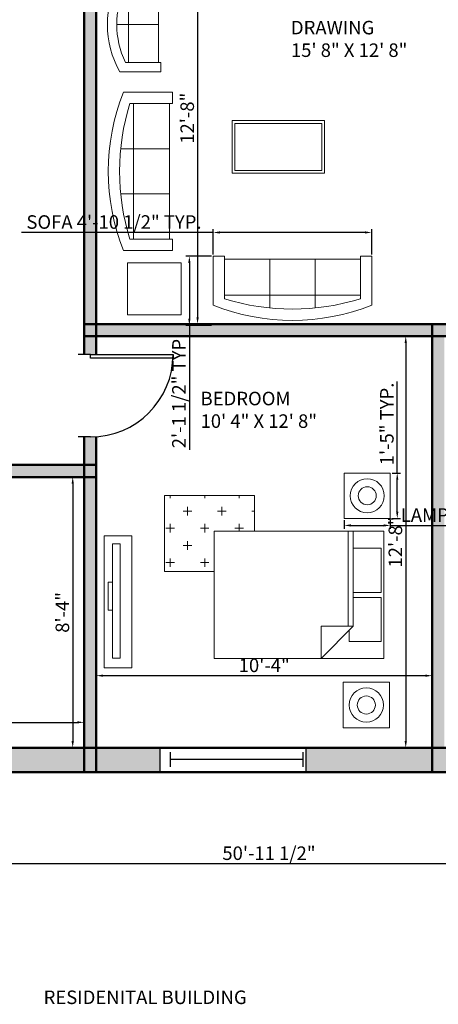
# Model space of a CAD drawing. Units: millimetres. Extents: x 3107 to 3757, y 777 to 1464.
# Tile 2 of 7: x 3324 to 3479, y 777 to 1140. Entities that reach past the tile are written whole.
import ezdxf

# ---------------------------------------------------------------- set-up
doc = ezdxf.new("R2010")
doc.units = ezdxf.units.MM
for name, color, linetype, lineweight in [('A-ANNO-DIMS', 50, 'Continuous', 18), ('A-ANNO-TEXT', 160, 'Continuous', 25), ('A-AREA-IDEN', 160, 'Continuous', 18), ('A-EQPM', 140, 'Continuous', 18), ('A-FURN-PATT', 140, 'Continuous', 13), ('A-WALL-PATT', 80, 'Continuous', 13), ('doors', 10, 'Continuous', 25), ('furniture', 140, 'Continuous', 18), ('walls', 80, 'Continuous', 50), ('windows', 30, 'Continuous', 25)]:
    doc.layers.add(name, color=color, linetype=linetype, lineweight=lineweight)
doc.styles.get("Standard").update_dxf_attribs({"font": 'arial.ttf'})
doc.dimstyles.new('ISO-25', dxfattribs={"dimtxt": 5, "dimasz": 2.5, "dimexe": 1.25, "dimexo": 0.625, "dimtad": 1, "dimdec": 0, "dimlunit": 3, "dimtxsty": 'Standard', "dimcen": 2.5, "dimadec": 0, "dimazin": 0, "dimtfac": 1, "dimtdec": 0, "dimtmove": 0, "dimatfit": 3, "dimfxl": 1, "dimarcsym": 0})

# ---------------------------------------------------------------- blocks, each defined once
blk = doc.blocks.new('*U2')
for p, q in [((0, 0), (0, -6)), ((40, 0), (40, -6))]:
    blk.add_line(p, q)
blk.add_lwpolyline([(0, 0), (0, 40), (1.75, 40), (1.75, 0)], close=True)
blk.add_arc((0, 0), 40, 0, 90)
blk = doc.blocks.new('*U4')
for p, q in [((0, 4), (0, 0)), ((36, 4), (36, 0)), ((0, 2), (36, 2))]:
    blk.add_line(p, q)
blk = doc.blocks.new('Sofa - Roundback 7 ft.')
for p, q in [((-12.00002, -32.4421), (-12.00003, -6.5971)), ((11.99997, -32.4421), (11.99998, -6.5971)), ((-36.000027, -34), (-36.000027, -11.4696)), ((-35.999844, -13.3819), (35.9998, -13.3819)), ((35.99998, -34), (35.99998, -11.4696)), ((-36.000027, -32.4421), (35.99998, -32.4421))]:
    blk.add_line(p, q)
for points in [[(-36.000027, -34), (-42.000027, -34), (-42.000027, -8)], [(41.99998, -8), (41.99998, -34), (35.99998, -34)]]:
    blk.add_lwpolyline(points)
for centre, radius, start, end in [((0, -114.25), 114.25, 68.43141, 111.5686), ((-0.00001, -127.1968), 121.1968, 72.72033, 107.2797)]:
    blk.add_arc(centre, radius, start, end)
blk = doc.blocks.new('Sofa - Roundback Loveseat 5 ft.')
for p, q in [((0, -32.44198), (0, -5.99998)), ((-24, -33.99998), (-24, -11.46958)), ((24.00004, -33.99998), (24.00004, -11.46958)), ((-23.9998, -13.38178), (23.99986, -13.38178)), ((-24, -32.44198), (24.00004, -32.44198))]:
    blk.add_line(p, q)
for points in [[(-24, -33.99998), (-30, -33.99998), (-30, -7.99998)], [(30.00004, -7.99998), (30.00004, -33.99998), (24.00004, -33.99998)]]:
    blk.add_lwpolyline(points)
for centre, radius, start, end in [((0, -60.24998), 60.24998, 60.13715, 119.8628), ((0, -61.38438), 55.38444, 64.32083, 115.6792)]:
    blk.add_arc(centre, radius, start, end)
blk = doc.blocks.new('Bed - Queen')
for p, q in [((0, -80.00003), (0, 0)), ((0, 0), (59.99999, 0)), ((59.99999, 0), (59.99999, -80.00003)), ((7.99999, -1.2), (28.79998, -1.2)), ((7.99999, -14.4), (7.99999, -1.2)), ((28.79998, -1.2), (28.79998, -14.4)), ((31.19999, -1.2), (51.99999, -1.2)), ((31.19999, -14.4), (31.19999, -1.2)), ((51.99999, -1.2), (51.99999, -16.4)), ((0, -14.4), (44.8, -14.4)), ((44.8, -16.8), (0, -16.8)), ((59.99999, -29.6), (44.8, -14.4)), ((44.8, -14.4), (44.8, -29.6)), ((51.99999, -16.4), (46.79936, -16.4)), ((44.8, -29.6), (59.99999, -29.6)), ((59.99999, -80.00003), (0, -80.00003))]:
    blk.add_line(p, q)
blk = doc.blocks.new('*D36')
at = {"layer": 'A-ANNO-DIMS', "color": 0, "lineweight": -2, "transparency": 16777216}
for p, q in [((3344.41, 971.43), (3345.04, 971.43)), ((3343.79, 968.93), (3343.79, 873.93)), ((3344.41, 871.43), (3345.04, 871.43))]:
    blk.add_line(p, q, dxfattribs=at)
at = {"layer": 'A-ANNO-DIMS', "color": 0, "transparency": 16777216}
for points in [[(3343.37, 968.93), (3344.21, 968.93), (3343.79, 971.43)], [(3343.37, 873.93), (3344.21, 873.93), (3343.79, 871.43)]]:
    blk.add_solid(points, dxfattribs=at)
at = {"layer": 'Defpoints', "color": 0, "transparency": 16777216}
for p in [(3343.79, 971.43), (3343.79, 871.43), (3343.79, 871.43)]:
    blk.add_point(p, dxfattribs=at)
at = {"layer": 'A-ANNO-DIMS', "color": 0, "transparency": 16777216, "insert": (3340.61, 921.43), "char_height": 5, "attachment_point": 5, "rotation": 90}
blk.add_mtext('8\'-4"', dxfattribs=at)
blk = doc.blocks.new('*D37')
at = {"layer": 'A-ANNO-DIMS', "color": 0, "lineweight": -2, "transparency": 16777216}
for p, q in [((3271.97, 881.46), (3271.97, 882.08)), ((3274.47, 880.83), (3345.47, 880.83)), ((3347.97, 881.46), (3347.97, 882.08))]:
    blk.add_line(p, q, dxfattribs=at)
at = {"layer": 'A-ANNO-DIMS', "color": 0, "transparency": 16777216}
for points in [[(3274.47, 881.25), (3274.47, 880.41), (3271.97, 880.83)], [(3345.47, 881.25), (3345.47, 880.41), (3347.97, 880.83)]]:
    blk.add_solid(points, dxfattribs=at)
at = {"layer": 'Defpoints', "color": 0, "transparency": 16777216}
for p in [(3271.97, 880.83), (3347.97, 880.83), (3347.97, 880.83)]:
    blk.add_point(p, dxfattribs=at)
at = {"layer": 'A-ANNO-DIMS', "color": 0, "transparency": 16777216, "insert": (3309.97, 884.01), "char_height": 5, "attachment_point": 5}
blk.add_mtext('6\'-4"', dxfattribs=at)
blk = doc.blocks.new('*D38')
at = {"layer": 'A-ANNO-DIMS', "color": 0, "lineweight": -2, "transparency": 16777216}
for p, q in [((3352.47, 899.15), (3352.47, 896.81)), ((3476.47, 899.15), (3476.47, 896.81)), ((3473.97, 898.06), (3354.97, 898.06))]:
    blk.add_line(p, q, dxfattribs=at)
at = {"layer": 'A-ANNO-DIMS', "color": 0, "transparency": 16777216}
for points in [[(3354.97, 898.48), (3354.97, 897.65), (3352.47, 898.06)], [(3473.97, 898.48), (3473.97, 897.65), (3476.47, 898.06)]]:
    blk.add_solid(points, dxfattribs=at)
at = {"layer": 'Defpoints', "color": 0, "transparency": 16777216}
for p in [(3352.47, 899.77), (3476.47, 899.77), (3352.47, 898.06)]:
    blk.add_point(p, dxfattribs=at)
at = {"layer": 'A-ANNO-DIMS', "color": 0, "transparency": 16777216, "insert": (3414.47, 901.24), "char_height": 5, "attachment_point": 5}
blk.add_mtext('10\'-4"', dxfattribs=at)
blk = doc.blocks.new('*D39')
at = {"layer": 'A-ANNO-DIMS', "color": 0, "lineweight": -2, "transparency": 16777216}
for p, q in [((3470.35, 1023.43), (3465.45, 1023.43)), ((3466.7, 1020.93), (3466.7, 873.93)), ((3472.66, 871.43), (3465.45, 871.43))]:
    blk.add_line(p, q, dxfattribs=at)
at = {"layer": 'A-ANNO-DIMS', "color": 0, "transparency": 16777216}
for points in [[(3466.28, 1020.93), (3467.12, 1020.93), (3466.7, 1023.43)], [(3466.28, 873.93), (3467.12, 873.93), (3466.7, 871.43)]]:
    blk.add_solid(points, dxfattribs=at)
at = {"layer": 'Defpoints', "color": 0, "transparency": 16777216}
for p in [(3470.97, 1023.43), (3466.7, 871.43), (3473.29, 871.43)]:
    blk.add_point(p, dxfattribs=at)
at = {"layer": 'A-ANNO-DIMS', "color": 0, "transparency": 16777216, "insert": (3463.52, 947.43), "char_height": 5, "attachment_point": 5, "rotation": 90}
blk.add_mtext('12\'-8"', dxfattribs=at)
blk = doc.blocks.new('*D40')
at = {"layer": 'A-ANNO-DIMS', "color": 0, "lineweight": -2, "transparency": 16777216}
for p, q in [((3385.8, 1179.93), (3391.12, 1179.93)), ((3389.87, 1177.43), (3389.87, 1030.43)), ((3384.41, 1027.93), (3391.12, 1027.93))]:
    blk.add_line(p, q, dxfattribs=at)
at = {"layer": 'A-ANNO-DIMS', "color": 0, "transparency": 16777216}
for points in [[(3389.45, 1177.43), (3390.29, 1177.43), (3389.87, 1179.93)], [(3389.45, 1030.43), (3390.29, 1030.43), (3389.87, 1027.93)]]:
    blk.add_solid(points, dxfattribs=at)
at = {"layer": 'Defpoints', "color": 0, "transparency": 16777216}
for p in [(3385.18, 1179.93), (3383.78, 1027.93), (3389.87, 1027.93)]:
    blk.add_point(p, dxfattribs=at)
at = {"layer": 'A-ANNO-DIMS', "color": 0, "transparency": 16777216, "insert": (3386.69, 1103.93), "char_height": 5, "attachment_point": 5, "rotation": 90}
blk.add_mtext('12\'-8"', dxfattribs=at)
blk = doc.blocks.new('BEDSIDE-TABLE-LAMP')
blk.add_lwpolyline([(17.05, 16.79), (0, 16.79), (0, 0), (17.05, 0)], close=True)
for radius in [6.29, 3.33]:
    blk.add_circle((8.52, 8.4), radius)
blk = doc.blocks.new('*D55')
at = {"layer": 'A-ANNO-DIMS', "color": 0, "lineweight": -2, "transparency": 16777216}
for p, q in [((3395.62, 1053.59), (3395.62, 1062.99)), ((3454.14, 1053.59), (3454.14, 1062.99)), ((3395.62, 1061.74), (3324.92, 1061.74)), ((3451.64, 1061.74), (3398.12, 1061.74))]:
    blk.add_line(p, q, dxfattribs=at)
at = {"layer": 'A-ANNO-DIMS', "color": 0, "transparency": 16777216}
for points in [[(3398.12, 1062.16), (3398.12, 1061.33), (3395.62, 1061.74)], [(3451.64, 1062.16), (3451.64, 1061.33), (3454.14, 1061.74)]]:
    blk.add_solid(points, dxfattribs=at)
at = {"layer": 'Defpoints', "color": 0, "transparency": 16777216}
for p in [(3395.62, 1061.74), (3395.62, 1052.96), (3454.14, 1052.96)]:
    blk.add_point(p, dxfattribs=at)
at = {"layer": 'A-ANNO-DIMS', "color": 0, "transparency": 16777216, "insert": (3359.02, 1064.95), "char_height": 5, "attachment_point": 5}
blk.add_mtext('SOFA 4\'-10 1/2" TYP.', dxfattribs=at)
blk = doc.blocks.new('*D56')
at = {"layer": 'A-ANNO-DIMS', "color": 0, "lineweight": -2, "transparency": 16777216}
for p, q in [((3394.99, 1052.96), (3385.59, 1052.96)), ((3386.84, 1050.46), (3386.84, 1029.92)), ((3394.99, 1027.42), (3385.59, 1027.42)), ((3386.84, 1027.42), (3386.84, 981.45))]:
    blk.add_line(p, q, dxfattribs=at)
at = {"layer": 'A-ANNO-DIMS', "color": 0, "transparency": 16777216}
for points in [[(3386.42, 1050.46), (3387.26, 1050.46), (3386.84, 1052.96)], [(3386.42, 1029.92), (3387.26, 1029.92), (3386.84, 1027.42)]]:
    blk.add_solid(points, dxfattribs=at)
at = {"layer": 'Defpoints', "color": 0, "transparency": 16777216}
for p in [(3395.62, 1052.96), (3386.84, 1027.42), (3395.62, 1027.42)]:
    blk.add_point(p, dxfattribs=at)
at = {"layer": 'A-ANNO-DIMS', "color": 0, "transparency": 16777216, "insert": (3383.63, 1003.19), "char_height": 5, "attachment_point": 5, "rotation": 90}
blk.add_mtext('2\'-1 1/2" TYP.', dxfattribs=at)
blk = doc.blocks.new('*D63')
at = {"layer": 'A-ANNO-DIMS', "color": 0, "lineweight": -2, "transparency": 16777216}
for p, q in [((3443.96, 955.48), (3443.96, 952.3)), ((3446.46, 953.55), (3458.5, 953.55)), ((3461, 955.48), (3461, 952.3)), ((3461, 953.55), (3515.97, 953.55))]:
    blk.add_line(p, q, dxfattribs=at)
at = {"layer": 'A-ANNO-DIMS', "color": 0, "transparency": 16777216}
for points in [[(3446.46, 953.96), (3446.46, 953.13), (3443.96, 953.55)], [(3458.5, 953.96), (3458.5, 953.13), (3461, 953.55)]]:
    blk.add_solid(points, dxfattribs=at)
at = {"layer": 'Defpoints', "color": 0, "transparency": 16777216}
for p in [(3443.96, 956.1), (3461, 956.1), (3461, 953.55)]:
    blk.add_point(p, dxfattribs=at)
at = {"layer": 'A-ANNO-DIMS', "color": 0, "transparency": 16777216, "insert": (3489.74, 956.72), "char_height": 5, "attachment_point": 5}
blk.add_mtext('LAMP 1\'-5" TYP.', dxfattribs=at)
blk = doc.blocks.new('*D64')
at = {"layer": 'A-ANNO-DIMS', "color": 0, "lineweight": -2, "transparency": 16777216}
for p, q in [((3463.56, 972.89), (3463.56, 1006.65)), ((3461.63, 972.89), (3464.81, 972.89)), ((3463.56, 958.6), (3463.56, 970.39)), ((3461.63, 956.1), (3464.81, 956.1))]:
    blk.add_line(p, q, dxfattribs=at)
at = {"layer": 'A-ANNO-DIMS', "color": 0, "transparency": 16777216}
for points in [[(3463.15, 970.39), (3463.98, 970.39), (3463.56, 972.89)], [(3463.15, 958.6), (3463.98, 958.6), (3463.56, 956.1)]]:
    blk.add_solid(points, dxfattribs=at)
at = {"layer": 'Defpoints', "color": 0, "transparency": 16777216}
for p in [(3461, 972.89), (3463.56, 972.89), (3461, 956.1)]:
    blk.add_point(p, dxfattribs=at)
at = {"layer": 'A-ANNO-DIMS', "color": 0, "transparency": 16777216, "insert": (3460.38, 991.02), "char_height": 5, "attachment_point": 5, "rotation": 90}
blk.add_mtext('1\'-5" TYP.', dxfattribs=at)
blk = doc.blocks.new('*D69')
at = {"layer": 'A-ANNO-DIMS', "color": 0, "lineweight": -2, "transparency": 16777216}
for p, q in [((3110.47, 861.8), (3110.47, 827.39)), ((3721.97, 861.8), (3721.97, 827.39)), ((3112.97, 828.64), (3719.47, 828.64))]:
    blk.add_line(p, q, dxfattribs=at)
at = {"layer": 'A-ANNO-DIMS', "color": 0, "transparency": 16777216}
for points in [[(3112.97, 829.06), (3112.97, 828.22), (3110.47, 828.64)], [(3719.47, 829.06), (3719.47, 828.22), (3721.97, 828.64)]]:
    blk.add_solid(points, dxfattribs=at)
at = {"layer": 'Defpoints', "color": 0, "transparency": 16777216}
for p in [(3110.47, 862.43), (3721.97, 862.43), (3721.97, 828.64)]:
    blk.add_point(p, dxfattribs=at)
at = {"layer": 'A-ANNO-DIMS', "color": 0, "transparency": 16777216, "insert": (3416.22, 831.85), "char_height": 5, "attachment_point": 5}
blk.add_mtext('50\'-11 1/2"', dxfattribs=at)

msp = doc.modelspace()

# ---------------------------------------------------------------- hatches: boundary and pattern name
at = {"layer": 'A-FURN-PATT'}
h = msp.add_hatch(dxfattribs=at)
h.set_pattern_fill('CROSS', color=256)
h.paths.add_polyline_path([(3395.95, 951.39), (3410.87, 951.39), (3410.87, 964.57), (3377.69, 964.57), (3377.69, 936.51), (3395.95, 936.51)])
at = {"layer": 'A-WALL-PATT'}
h = msp.add_hatch(color=256, dxfattribs=at)
h.dxf.hatch_style = 1
h.paths.add_polyline_path([(3119.47, 1087.39), (3110.47, 1087.39), (3110.47, 1027.93), (3119.47, 1027.93)])
h.paths.add_polyline_path([(3119.47, 1027.93), (3110.47, 1027.93), (3110.47, 1023.43), (3119.47, 1023.43)])
h.paths.add_polyline_path([(3267.47, 1027.93), (3119.47, 1027.93), (3119.47, 1023.43), (3267.47, 1023.43)])
h.paths.add_polyline_path([(3119.47, 1023.43), (3110.47, 1023.43), (3110.47, 979.44), (3119.47, 979.44)])
h.paths.add_polyline_path([(3299.97, 1179.93), (3295.47, 1179.93), (3295.47, 1027.93), (3299.97, 1027.93)])
h.paths.add_polyline_path([(3295.47, 1027.93), (3271.97, 1027.93), (3271.97, 1023.43), (3295.47, 1023.43)])
h.paths.add_polyline_path([(3271.97, 1027.93), (3267.47, 1027.93), (3267.47, 1023.43), (3271.97, 1023.43)])
h.paths.add_polyline_path([(3299.97, 1027.93), (3295.47, 1027.93), (3295.47, 1023.43), (3299.97, 1023.43)])
h.paths.add_polyline_path([(3299.97, 1184.43), (3295.47, 1184.43), (3295.47, 1179.93), (3299.97, 1179.93)])
h.paths.add_polyline_path([(3295.47, 1184.43), (3288.38, 1184.43), (3288.38, 1182.47), (3288.38, 1179.93), (3295.47, 1179.93)])
h.paths.add_polyline_path([(3352.47, 1179.93), (3347.97, 1179.93), (3347.97, 1027.93), (3352.47, 1027.93)])
h.paths.add_polyline_path([(3352.47, 1184.43), (3347.97, 1184.43), (3347.97, 1179.93), (3352.47, 1179.93)])
h.paths.add_polyline_path([(3464.47, 1184.43), (3352.47, 1184.43), (3352.47, 1179.93), (3464.47, 1179.93)])
h.paths.add_polyline_path([(3468.97, 1288.93), (3464.47, 1288.93), (3464.47, 1184.43), (3468.97, 1184.43)])
h.paths.add_polyline_path([(3468.97, 1184.43), (3464.47, 1184.43), (3464.47, 1179.93), (3468.97, 1179.93)])
h.paths.add_polyline_path([(3195.97, 1248.43), (3191.47, 1248.43), (3191.47, 1184.43), (3195.97, 1184.43)])
h.paths.add_polyline_path([(3195.97, 1184.43), (3191.47, 1184.43), (3191.47, 1179.93), (3195.97, 1179.93)])
h.paths.add_polyline_path([(3191.47, 1184.43), (3183.28, 1184.43), (3183.28, 1181.58), (3183.28, 1179.93), (3191.47, 1179.93)])
h.paths.add_polyline_path([(3243.97, 1184.43), (3195.97, 1184.43), (3195.97, 1179.93), (3243.97, 1179.93)])
h.paths.add_polyline_path([(3257.91, 1182.47), (3257.91, 1184.43), (3248.47, 1184.43), (3248.47, 1179.93), (3258.02, 1179.93, -0.020891)])
h.paths.add_polyline_path([(3248.47, 1184.43), (3243.97, 1184.43), (3243.97, 1179.93), (3248.47, 1179.93)])
h.paths.add_polyline_path([(3248.47, 1189.24), (3247.51, 1189.24), (3243.97, 1189.24), (3243.97, 1184.43), (3248.47, 1184.43)])
h.paths.add_polyline_path([(3166.87, 1184.43), (3119.47, 1184.43), (3119.47, 1179.93), (3166.63, 1179.93), (3166.63, 1181.58, -0.042981)])
h.paths.add_polyline_path([(3119.47, 1184.43), (3110.47, 1184.43), (3110.47, 1179.93), (3119.47, 1179.93)])
h.paths.add_polyline_path([(3119.47, 1248.43), (3110.47, 1248.43), (3110.47, 1184.43), (3119.47, 1184.43)])
h.paths.add_polyline_path([(3119.47, 1179.93), (3110.47, 1179.93), (3110.47, 1140.65), (3119.47, 1140.65)])
h.paths.add_polyline_path([(3119.47, 1288.93), (3110.47, 1288.93), (3110.47, 1252.93), (3119.47, 1252.93)])
h.paths.add_polyline_path([(3119.47, 1252.93), (3110.47, 1252.93), (3110.47, 1248.43), (3119.47, 1248.43)])
h.paths.add_polyline_path([(3191.47, 1252.93), (3119.47, 1252.93), (3119.47, 1248.43), (3191.47, 1248.43)])
h.paths.add_polyline_path([(3195.97, 1288.93), (3191.47, 1288.93), (3191.47, 1252.93), (3195.97, 1252.93)])
h.paths.add_polyline_path([(3195.97, 1252.93), (3191.47, 1252.93), (3191.47, 1248.43), (3195.97, 1248.43)])
h.paths.add_polyline_path([(3248.47, 1293.43), (3243.97, 1293.43), (3243.97, 1288.93), (3248.47, 1288.93)])
h.paths.add_polyline_path([(3243.97, 1293.43), (3195.97, 1293.43), (3195.97, 1288.93), (3243.97, 1288.93)])
h.paths.add_polyline_path([(3303.47, 1293.43), (3248.47, 1293.43), (3248.47, 1288.93), (3303.47, 1288.93)])
h.paths.add_polyline_path([(3248.47, 1288.93), (3243.97, 1288.93), (3243.97, 1205.51, -0.053712), (3247.51, 1205.89), (3248.47, 1205.89)])
h.paths.add_polyline_path([(3191.47, 1293.43), (3119.47, 1293.43), (3119.47, 1288.93), (3191.47, 1288.93)])
h.paths.add_polyline_path([(3119.47, 1293.43), (3110.47, 1293.43), (3110.47, 1288.93), (3119.47, 1288.93)])
h.paths.add_polyline_path([(3119.47, 1322.96, -0.065064), (3111.64, 1321.93), (3110.47, 1321.93), (3110.47, 1293.43), (3119.47, 1293.43)])
h.paths.add_polyline_path([(3195.97, 1293.43), (3191.47, 1293.43), (3191.47, 1288.93), (3195.97, 1288.93)])
h.paths.add_polyline_path([(3119.47, 1450.43), (3110.47, 1450.43), (3110.47, 1441.43), (3119.47, 1441.43)])
h.paths.add_polyline_path([(3119.47, 1441.43), (3110.47, 1441.43), (3110.47, 1352.4), (3111.64, 1352.4), (3119.47, 1352.4)])
h.paths.add_polyline_path([(3176.58, 1450.43), (3119.47, 1450.43), (3119.47, 1441.43), (3176.58, 1441.43)])
h.paths.add_polyline_path([(3323.19, 1450.43), (3307.97, 1450.43), (3307.97, 1441.43), (3323.19, 1441.43)])
h.paths.add_polyline_path([(3307.97, 1450.43), (3303.47, 1450.43), (3303.47, 1441.43), (3307.97, 1441.43)])
h.paths.add_polyline_path([(3303.47, 1450.43), (3229.4, 1450.43), (3229.4, 1441.43), (3303.47, 1441.43)])
h.paths.add_polyline_path([(3307.97, 1441.43), (3303.47, 1441.43), (3303.47, 1363.43), (3307.97, 1363.43)])
h.paths.add_polyline_path([(3307.97, 1363.43), (3303.47, 1363.43), (3303.47, 1358.93), (3307.97, 1358.93)])
h.paths.add_polyline_path([(3307.97, 1358.93), (3303.47, 1358.93), (3303.47, 1342.3), (3305.5, 1342.3, -0.037178), (3307.97, 1342.12)])
h.paths.add_polyline_path([(3379.97, 1363.43), (3307.97, 1363.43), (3307.97, 1358.93), (3379.97, 1358.93)])
h.paths.add_polyline_path([(3384.47, 1393.61), (3383.04, 1393.61), (3379.97, 1393.61), (3379.97, 1363.43), (3384.47, 1363.43)])
h.paths.add_polyline_path([(3384.47, 1363.43), (3379.97, 1363.43), (3379.97, 1358.93), (3384.47, 1358.93)])
h.paths.add_polyline_path([(3384.47, 1358.93), (3379.97, 1358.93), (3379.97, 1293.43), (3384.47, 1293.43)])
h.paths.add_polyline_path([(3384.47, 1441.43), (3379.97, 1441.43), (3379.97, 1409.98, -0.046389), (3383.04, 1410.27), (3384.47, 1410.27)])
h.paths.add_polyline_path([(3384.47, 1450.43), (3379.97, 1450.43), (3379.97, 1441.43), (3384.47, 1441.43)])
h.paths.add_polyline_path([(3379.97, 1450.43), (3357.18, 1450.43), (3357.18, 1441.43), (3379.97, 1441.43)])
h.paths.add_polyline_path([(3432.79, 1450.43), (3384.47, 1450.43), (3384.47, 1441.43), (3432.79, 1441.43)])
h.paths.add_polyline_path([(3540.47, 1450.43), (3484.18, 1450.43), (3484.18, 1441.43), (3540.47, 1441.43)])
h.paths.add_polyline_path([(3544.97, 1450.43), (3540.47, 1450.43), (3540.47, 1441.43), (3544.97, 1441.43)])
h.paths.add_polyline_path([(3544.97, 1441.43), (3540.47, 1441.43), (3540.47, 1293.43), (3544.97, 1293.43)])
h.paths.add_polyline_path([(3590.83, 1450.43), (3544.97, 1450.43), (3544.97, 1441.43), (3590.83, 1441.43)])
h.paths.add_polyline_path([(3712.97, 1450.43), (3645.62, 1450.43), (3645.62, 1441.43), (3712.97, 1441.43)])
h.paths.add_polyline_path([(3721.97, 1441.43), (3712.97, 1441.43), (3712.97, 1288.93), (3712.97, 1184.43), (3721.97, 1184.43), (3721.97, 1288.93)])
h.paths.add_polyline_path([(3721.97, 1450.43), (3712.97, 1450.43), (3712.97, 1441.43), (3721.97, 1441.43)])
h.paths.add_polyline_path([(3712.97, 1184.43), (3658.24, 1184.43), (3658.24, 1183.15), (3658.24, 1179.93), (3712.97, 1179.93)])
h.paths.add_polyline_path([(3721.97, 1184.43), (3712.97, 1184.43), (3712.97, 1179.93), (3721.97, 1179.93)])
h.paths.add_polyline_path([(3597.32, 1183.15), (3597.32, 1184.43), (3544.97, 1184.43), (3544.97, 1179.93), (3597.32, 1179.93)])
h.paths.add_polyline_path([(3544.97, 1184.43), (3540.47, 1184.43), (3540.47, 1179.93), (3544.97, 1179.93)])
h.paths.add_polyline_path([(3544.97, 1179.93), (3540.47, 1179.93), (3540.47, 1143.69), (3543.65, 1143.69), (3544.97, 1143.69)])
h.paths.add_polyline_path([(3721.97, 1179.93), (3712.97, 1179.93), (3712.97, 1006.22), (3712.97, 871.43), (3721.97, 871.43), (3721.97, 1006.22)])
h.paths.add_polyline_path([(3468.97, 1293.43), (3464.47, 1293.43), (3464.47, 1288.93), (3468.97, 1288.93)])
h.paths.add_polyline_path([(3540.47, 1293.43), (3468.97, 1293.43), (3468.97, 1288.93), (3540.47, 1288.93)])
h.paths.add_polyline_path([(3544.97, 1293.43), (3540.47, 1293.43), (3540.47, 1288.93), (3544.97, 1288.93)])
h.paths.add_polyline_path([(3464.47, 1293.43), (3417.83, 1293.43, -0.015057), (3417.88, 1291.6), (3417.88, 1288.93), (3464.47, 1288.93)])
h.paths.add_polyline_path([(3379.97, 1293.43), (3307.97, 1293.43), (3307.97, 1288.93), (3379.97, 1288.93)])
h.paths.add_polyline_path([(3307.97, 1325.65), (3305.5, 1325.65), (3303.47, 1325.65), (3303.47, 1293.43), (3307.97, 1293.43)])
h.paths.add_polyline_path([(3307.97, 1293.43), (3303.47, 1293.43), (3303.47, 1288.93), (3307.97, 1288.93)])
h.paths.add_polyline_path([(3384.47, 1293.43), (3379.97, 1293.43), (3379.97, 1288.93), (3384.47, 1288.93)])
h.paths.add_polyline_path([(3387.42, 1291.6), (3387.42, 1293.43), (3384.47, 1293.43), (3384.47, 1288.93), (3387.42, 1288.93)])
h.paths.add_polyline_path([(3119.47, 927.28), (3110.47, 927.28), (3110.47, 871.43), (3119.47, 871.43)])
h.paths.add_polyline_path([(3119.47, 871.43), (3110.47, 871.43), (3110.47, 862.43), (3119.47, 862.43)])
h.paths.add_polyline_path([(3267.47, 871.43), (3119.47, 871.43), (3119.47, 862.43), (3267.47, 862.43)])
h.paths.add_polyline_path([(3271.97, 971.43), (3267.47, 971.43), (3267.47, 871.43), (3271.97, 871.43)])
h.paths.add_polyline_path([(3271.97, 871.43), (3267.47, 871.43), (3267.47, 862.43), (3271.97, 862.43)])
h.paths.add_polyline_path([(3287.13, 871.43), (3271.97, 871.43), (3271.97, 862.43), (3287.13, 862.43)])
h.paths.add_polyline_path([(3347.97, 871.43), (3318.96, 871.43), (3318.96, 862.43), (3347.97, 862.43)])
h.paths.add_polyline_path([(3352.47, 971.43), (3347.97, 971.43), (3347.97, 871.43), (3352.47, 871.43)])
h.paths.add_polyline_path([(3352.47, 871.43), (3347.97, 871.43), (3347.97, 862.43), (3352.47, 862.43)])
h.paths.add_polyline_path([(3375.96, 871.43), (3352.47, 871.43), (3352.47, 862.43), (3375.96, 862.43)])
h.paths.add_polyline_path([(3352.47, 975.93), (3347.97, 975.93), (3347.97, 971.43), (3352.47, 971.43)])
h.paths.add_polyline_path([(3352.47, 986.27, -0.01722), (3350.37, 986.2), (3347.97, 986.2), (3347.97, 975.93), (3352.47, 975.93)])
h.paths.add_polyline_path([(3347.97, 975.93), (3292.38, 975.93), (3292.38, 973.47, -0.030785), (3292.25, 971.43), (3347.97, 971.43)])
h.paths.add_polyline_path([(3271.97, 985.98), (3269.95, 985.98), (3267.47, 985.98), (3267.47, 975.93), (3271.97, 975.93)])
h.paths.add_polyline_path([(3271.97, 975.93), (3267.47, 975.93), (3267.47, 971.43), (3271.97, 971.43)])
h.paths.add_polyline_path([(3275.72, 975.93), (3271.97, 975.93), (3271.97, 971.43), (3275.72, 971.43), (3275.72, 973.47)])
h.paths.add_polyline_path([(3271.97, 1023.43), (3267.47, 1023.43), (3267.47, 1016.34, -0.020418), (3269.95, 1016.44), (3271.97, 1016.44)])
h.paths.add_polyline_path([(3352.47, 1023.43), (3347.97, 1023.43), (3347.97, 1016.67), (3350.37, 1016.67), (3352.47, 1016.67)])
h.paths.add_polyline_path([(3352.47, 1027.93), (3347.97, 1027.93), (3347.97, 1023.43), (3352.47, 1023.43)])
h.paths.add_polyline_path([(3476.47, 1027.93), (3352.47, 1027.93), (3352.47, 1023.43), (3476.47, 1023.43)])
h.paths.add_polyline_path([(3540.47, 1027.93), (3480.97, 1027.93), (3480.97, 1023.43), (3540.47, 1023.43)])
h.paths.add_polyline_path([(3480.97, 1027.93), (3476.47, 1027.93), (3476.47, 1023.43), (3480.97, 1023.43)])
h.paths.add_polyline_path([(3480.97, 1023.43), (3476.47, 1023.43), (3476.47, 871.43), (3480.97, 871.43)])
h.paths.add_polyline_path([(3476.47, 871.43), (3429.88, 871.43), (3429.88, 862.43), (3476.47, 862.43)])
h.paths.add_polyline_path([(3480.97, 871.43), (3476.47, 871.43), (3476.47, 862.43), (3480.97, 862.43)])
h.paths.add_polyline_path([(3493.81, 871.43), (3480.97, 871.43), (3480.97, 862.43), (3493.81, 862.43)])
h.paths.add_polyline_path([(3712.97, 871.43), (3525.61, 871.43), (3525.61, 862.43), (3712.97, 862.43)])
h.paths.add_polyline_path([(3721.97, 871.43), (3712.97, 871.43), (3712.97, 862.43), (3721.97, 862.43)])

# ---------------------------------------------------------------- linework, layer by layer
at = {"layer": 'A-EQPM'}
for points in [[(3355.44, 949.76), (3365.61, 949.76), (3365.61, 901), (3355.44, 901)], [(3358.52, 946.76), (3361.24, 946.76), (3361.24, 904.54), (3358.52, 904.54)], [(3358.52, 932.58), (3356.93, 932.58), (3356.93, 922.22), (3358.52, 922.22)]]:
    msp.add_lwpolyline(points, close=True, dxfattribs=at)
at = {"layer": 'furniture'}
for p, q in [((3377.69, 936.51), (3377.69, 964.57)), ((3377.69, 964.57), (3410.87, 964.57)), ((3410.87, 964.57), (3410.87, 951.39)), ((3395.95, 936.51), (3377.69, 936.51))]:
    msp.add_line(p, q, dxfattribs=at)
for points in [[(3402.68, 1083.63), (3402.68, 1103.03), (3436.67, 1103.03), (3436.67, 1083.63)], [(3403.68, 1084.63), (3403.68, 1102.03), (3435.67, 1102.03), (3435.67, 1084.63)], [(3363.99, 1050.54), (3383.78, 1050.54), (3383.78, 1031.32), (3363.99, 1031.32)]]:
    msp.add_lwpolyline(points, close=True, dxfattribs=at)
at = {"layer": 'walls'}
for p, q in [((3347.97, 1184.43), (3347.97, 1016.67)), ((3352.47, 1184.43), (3352.47, 1016.67)), ((3347.97, 1027.93), (3544.97, 1027.93)), ((3476.47, 1027.93), (3476.47, 862.43)), ((3347.97, 1023.43), (3544.97, 1023.43)), ((3347.97, 986.2), (3347.97, 862.43)), ((3352.47, 986.27), (3352.47, 862.43)), ((3292.38, 975.93), (3352.47, 975.93)), ((3292.25, 971.43), (3352.47, 971.43)), ((3110.47, 871.43), (3721.97, 871.43)), ((3110.47, 862.43), (3721.97, 862.43))]:
    msp.add_line(p, q, dxfattribs=at)
at = {"layer": 'windows'}
for p, q in [((3375.96, 871.43), (3375.96, 862.43)), ((3429.88, 871.43), (3429.88, 862.43))]:
    msp.add_line(p, q, dxfattribs=at)

# ---------------------------------------------------------------- block references
at = {"layer": 'doors', "xscale": 0.7615706373352984, "yscale": 0.7615706373352984, "zscale": 0.7615706373352984, "rotation": 269.9999999999999}
msp.add_blockref('*U2', (3350.37, 1016.67), dxfattribs=at)
at = {"layer": 'furniture'}
for name, p, xscale, yscale, zscale, rotation in [('Sofa - Roundback Loveseat 5 ft.', (3356.57, 1138.5), 0.5809767439628069, 0.5809767439628069, 0.5809767439628069, 89.99996919953323), ('Sofa - Roundback 7 ft.', (3356.91, 1084.32), 0.6967080671381904, 0.6967080671381904, 0.6967080671381904, 90), ('Sofa - Roundback 7 ft.', (3424.88, 1029.28), 0.6967080671381904, 0.6967080671381904, 0.6967080671381904, 180), ('Bed - Queen', (3458.63, 951.39), 0.7835133119924312, 0.7835133119924312, 0.7835133119924312, 270)]:
    msp.add_blockref(name, p, dxfattribs=dict(at, xscale=xscale, yscale=yscale, zscale=zscale, rotation=rotation))
for p in [(3443.96, 956.1), (3443.63, 878.83)]:
    msp.add_blockref('BEDSIDE-TABLE-LAMP', p, dxfattribs=at)
at = {"layer": 'windows', "xscale": 1.357941570966636, "yscale": 1.357941570966636, "zscale": 1.357941570966636, "rotation": 180}
msp.add_blockref('*U4', (3428.79, 869.87), dxfattribs=at)

# ---------------------------------------------------------------- texts
at = {"layer": 'A-ANNO-TEXT', "insert": (3333.05, 781.79), "char_height": 5, "attachment_point": 1}
msp.add_mtext_dynamic_manual_height_columns('RESIDENITAL BUILDING ', width=274.8882, gutter_width=12.5, heights=[0], dxfattribs=at)
at = {"layer": 'A-AREA-IDEN', "char_height": 5, "attachment_point": 1}
for s, width, insert in [('DRAWING \\P15\' 8" X 12\' 8"', 62.5375, (3424.32, 1139.89)), ('BEDROOM\\P10\' 4" X 12\' 8"', 61.2307, (3390.97, 1002.91))]:
    msp.add_mtext_dynamic_manual_height_columns(s, width=width, gutter_width=12.5, heights=[0], dxfattribs=dict(at, insert=insert))

# ---------------------------------------------------------------- dimensions: what is measured, and where the dimension line sits
at = {"layer": 'A-ANNO-DIMS'}
for base, p1, p2, picture, middle in [((3389.87, 1027.93), (3385.18, 1179.93), (3383.78, 1027.93), '*D40', (3386.69, 1103.93)), ((3466.7, 871.43), (3470.97, 1023.43), (3473.29, 871.43), '*D39', (3463.52, 947.43)), ((3343.79, 871.43), (3343.79, 971.43), (3343.79, 871.43), '*D36', (3340.61, 921.43))]:
    dim = msp.add_linear_dim(base=base, p1=p1, p2=p2, angle=90, dimstyle='ISO-25', override={"dimclrd": 0, "dimclre": 0, "dimclrt": 0}, dxfattribs=at)
    dim.commit()
    dim.dimension.update_dxf_attribs({"geometry": picture, "text_midpoint": middle})
for base, p1, p2, angle, text, picture, middle in [((3395.62, 1061.74), (3454.14, 1052.96), (3395.62, 1052.96), 180, 'SOFA <> TYP.', '*D55', (3359.02, 1064.95)), ((3386.84, 1027.42), (3395.62, 1052.96), (3395.62, 1027.42), 270, '<> TYP.', '*D56', (3383.63, 1003.19)), ((3463.56, 972.89), (3461, 956.1), (3461, 972.89), 90, '<> TYP.', '*D64', (3460.38, 991.02))]:
    dim = msp.add_linear_dim(base=base, p1=p1, p2=p2, angle=angle, text=text, dimstyle='ISO-25', override={"dimdec": 1, "dimlfac": 1, "dimrnd": 0, "dimzin": 1, "dimdsep": 46, "dimlunit": 4, "dimfrac": 2}, dxfattribs=at)
    dim.commit()
    dim.dimension.update_dxf_attribs({"geometry": picture, "text_midpoint": middle})
dim = msp.add_linear_dim(base=(3461, 953.55), p1=(3443.96, 956.1), p2=(3461, 956.1), text='LAMP <> TYP.', dimstyle='ISO-25', override={"dimdec": 1, "dimlfac": 1, "dimrnd": 0, "dimzin": 1, "dimdsep": 46, "dimlunit": 4, "dimfrac": 2}, dxfattribs=at)
dim.commit()
dim.dimension.update_dxf_attribs({"geometry": '*D63', "text_midpoint": (3489.74, 956.72)})
for base, p1, p2, override, picture, middle in [((3352.47, 898.06), (3476.47, 899.77), (3352.47, 899.77), {"dimclrd": 0, "dimclre": 0, "dimclrt": 0}, '*D38', (3414.47, 901.24)), ((3347.97, 880.83), (3271.97, 880.83), (3347.97, 880.83), {"dimclrd": 0, "dimclre": 0, "dimclrt": 0}, '*D37', (3309.97, 884.01)), ((3721.97, 828.64), (3110.47, 862.43), (3721.97, 862.43), {"dimdec": 1, "dimlfac": 1, "dimrnd": 0, "dimzin": 1, "dimdsep": 46, "dimlunit": 4, "dimfrac": 2}, '*D69', (3416.22, 831.85))]:
    dim = msp.add_linear_dim(base=base, p1=p1, p2=p2, dimstyle='ISO-25', override=override, dxfattribs=at)
    dim.commit()
    dim.dimension.update_dxf_attribs({"geometry": picture, "text_midpoint": middle})

doc.saveas('drawing.dxf')
